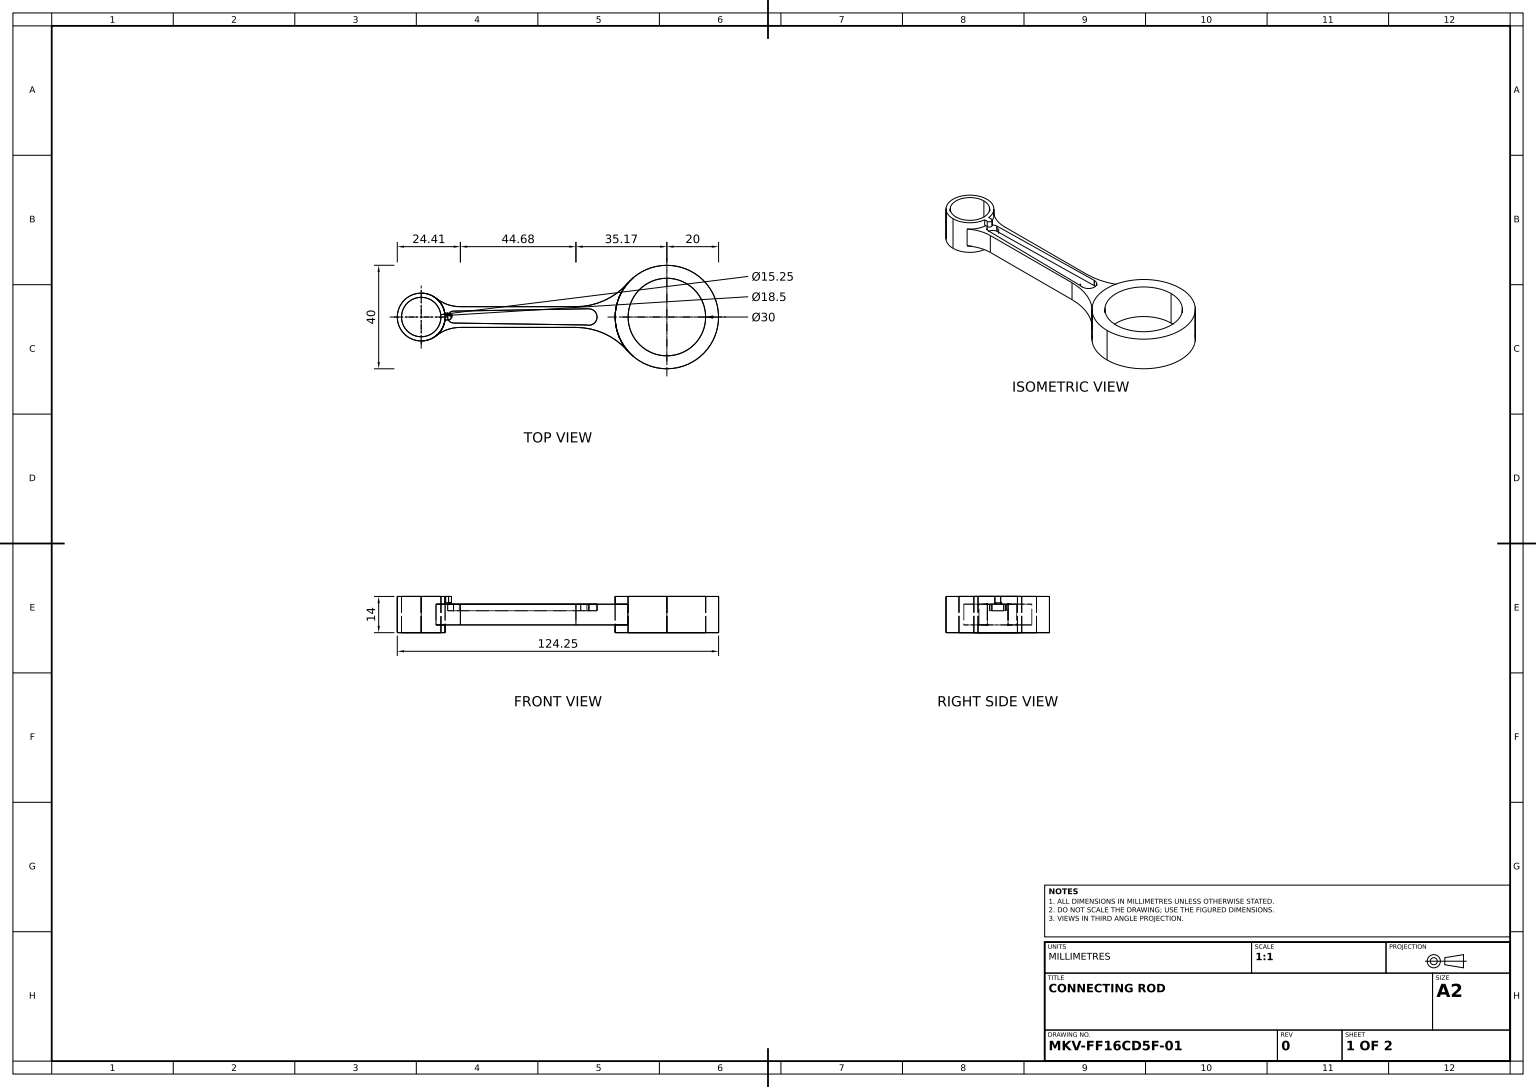
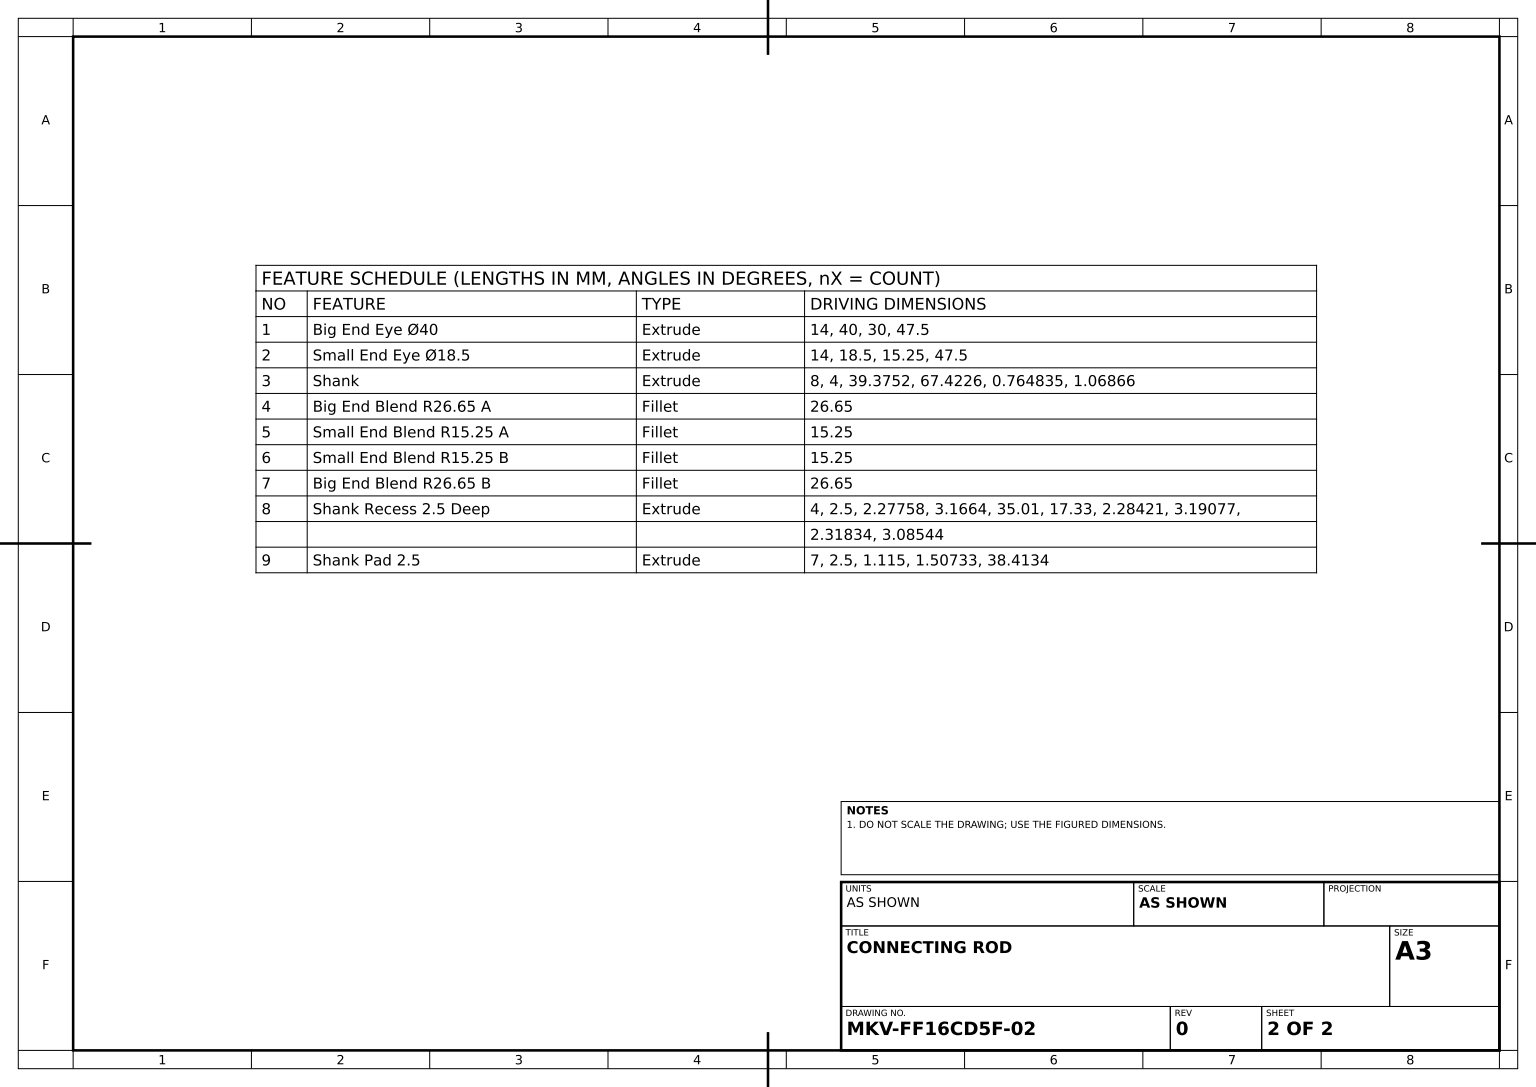
SolidWorks part; units mm, degrees
material "Plain Carbon Steel"
ref_plane "Front Plane" through (0, 0, 0) normal (0, 0, 1) x (1, 0, 0)
ref_plane "Top Plane" through (0, 0, 0) normal (0, 1, 0) x (1, 0, 0)
ref_plane "Right Plane" through (0, 0, 0) normal (1, 0, 0) x (0, 0, -1)
sketch "Big End Eye Sketch" plane through (0, 0, 0) normal (0, 1, 0) x (1, 0, 0)
  line L0 (0, 0) -> (47.5, 0)
  circle A0 centre (47.5, 0) radius 20
  circle A1 centre (47.5, 0) radius 15
  dimension "D1" = 40
  dimension "D2" = 30
  dimension "D3" = 47.5
extrude "Big End Eye Ø40" add sketch "Big End Eye Sketch" along normal mid plane 14
sketch "Small End Eye Sketch" plane through (0, 0, 0) normal (0, 1, 0) x (1, 0, 0)
  line L0 (0, 0) -> (-47.5, 0)
  circle A0 centre (-47.5, 0) radius 9.25
  circle A1 centre (-47.5, 0) radius 7.625
  dimension "D1" = 18.5
  dimension "D2" = 15.25
  dimension "D3" = 47.5
extrude "Small End Eye Ø18.5" add sketch "Small End Eye Sketch" along normal mid plane 14 separate body
sketch "Shank Profile Sketch" plane through (0, 0, 0) normal (0, 1, 0) x (1, 0, 0)
  line L2 (27.2826, 4) -> (28.0474, 4)
  line L3 (27.2826, 4) -> (-39.3752, 4)
  line L5 (-38.3065, -4) -> (28.0474, -4)
  line L6 (28.0474, -4) -> (28.0474, 4)
  line L7 (-39.3752, 4) -> (-39.3752, -4)
  line L8 (-39.3752, -4) -> (-38.3065, -4)
  dimension "D1" = 8
  dimension "D2" = 4
  dimension "D3" = 39.3752
  dimension "D4" = 67.4226
  dimension "D5" = 0.7648
  dimension "D6" = 1.0687
extrude "Shank" add sketch "Shank Profile Sketch" along normal mid plane 8
fillet "Big End Blend R26.65 A" radius 26.65 1 edges at (27.9041, 0, -4)
fillet "Small End Blend R15.25 A" radius 15.25 1 edges at (-39.1596, 0, -4)
fillet "Small End Blend R15.25 B" radius 15.25 1 edges at (-39.1596, 0, 4)
fillet "Big End Blend R26.65 B" radius 26.65 1 edges at (27.9041, 0, 4)
ref_plane "Plane1" through (0, 4, 0) normal (0, 1, 0) x (1, 0, 0)
sketch "Shank Recess Sketch" plane through (0, 4, 0) normal (0, 1, 0) x (1, 0, 0)
  line L0 (-35.01, -2.2776) -> (-35.01, -2.3183)
  line L2 (17.33, 3.1664) -> (17.33, 3.1908)
  line L3 (17.33, 3.1908) -> (-35.01, 2.2842)
  line L4 (-35.01, 2.2842) -> (-35.01, 2.2776)
  line L5 (-35.01, -2.3183) -> (17.33, -3.0854)
  arc A0 (-35.01, 2.2776) -> (-35.01, -2.2776) centre (-35.01, 0) ccw
  arc A1 (16.572, -3.0743) -> (17.33, 3.1664) centre (17.33, 0) ccw
  dimension "D1" = 2.2776
  dimension "D2" = 3.1664
  dimension "D3" = 35.01
  dimension "D4" = 17.33
  dimension "D5" = 2.2842
  dimension "D6" = 3.1908
  dimension "D7" = 2.3183
  dimension "D8" = 3.0854
extrude "Shank Recess 2.5 Deep" cut sketch "Shank Recess Sketch" against normal blind 2.5
ref_plane "Plane2" through (0, 7, 0) normal (0, 1, 0) x (1, 0, 0)
sketch "Shank Pad Sketch" plane through (0, 7, 0) normal (0, 1, 0) x (1, 0, 0)
  line L0 (0, 0) -> (-38.4134, 0)
  line L1 (-38.4134, 0) -> (-36.9061, 0)
  line L2 (-36.9061, 1.115) -> (-38.4134, 1.115)
  line L3 (-38.4134, 1.115) -> (-38.4134, -1.115)
  line L4 (-38.4134, -1.115) -> (-36.9061, -1.115)
  arc A0 (-36.9061, -1.115) -> (-36.9061, 1.115) centre (-36.9061, 0) ccw
  dimension "D1" = 1.115
  dimension "D2" = 1.5073
  dimension "D3" = 38.4134
extrude "Shank Pad 2.5" add sketch "Shank Pad Sketch" against normal blind 2.5 contours L0 A0 L2 L3 | L4 A0 L0 L3
